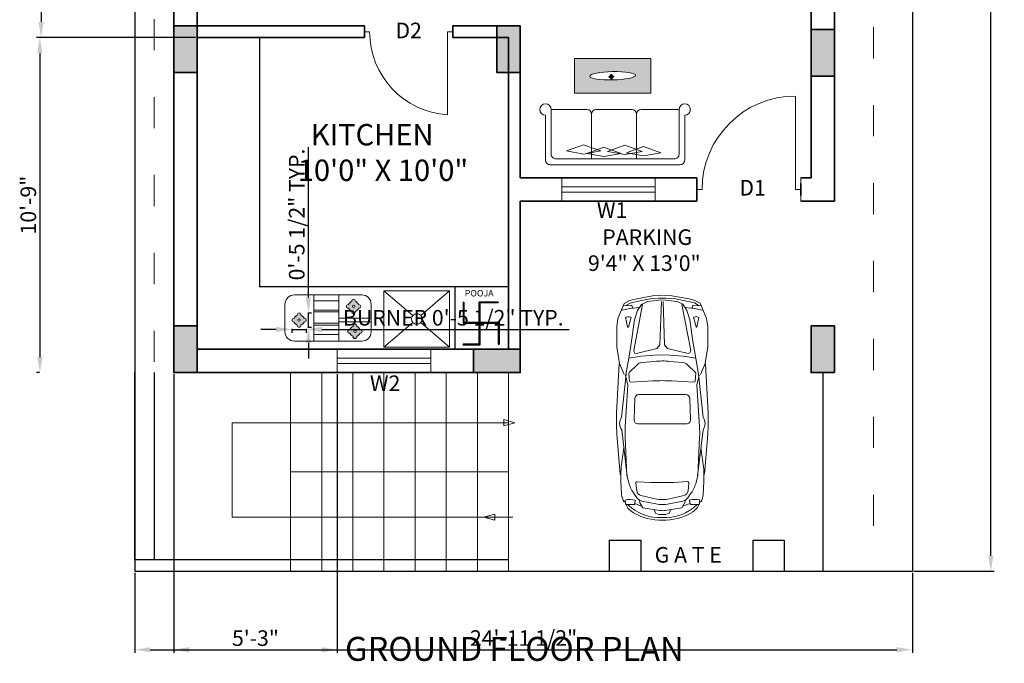
# Model space of a CAD drawing. Units: inches. Extents: x 40559 to 41508, y 131086 to 132358.
# Tile 1 of 5: x 40560 to 40939, y 131086 to 131334. Entities that reach past the tile are written whole.
import ezdxf

# ---------------------------------------------------------------- set-up
doc = ezdxf.new("R2010")
doc.units = ezdxf.units.IN
doc.linetypes.add('ACAD_ISO03W100', pattern=[30, 12, -18])
for name, color, linetype, lineweight in [('A-ANNO-DIMS', 2, 'Continuous', 18), ('A-ANNO-TEXT', 7, 'Continuous', 18), ('A-ANNO-TITL', 7, 'Continuous', 25), ('A-AREA-IDEN', 7, 'Continuous', 18), ('A-EQPM', 4, 'Continuous', 18), ('A-FLOR-CASE', 7, 'Continuous', 25), ('A-FLOR-FIXT', 4, 'Continuous', 18), ('A-FLOR-OVHD', 240, 'ACAD_ISO03W100', 13), ('A-FLOR-STRS', 240, 'Continuous', 18), ('A-FURN', 9, 'Continuous', 18), ('A-FURN-PATT', 252, 'Continuous', 13), ('A-SITE-VEHI', 9, 'Continuous', 13), ('A-SITE-WALL', 7, 'Continuous', 30), ('A-WALL', 7, 'Continuous', 35), ('C-PROP', 7, 'Continuous', 25), ('Doors', 50, 'Continuous', 18), ('Windows', 70, 'Continuous', 18)]:
    doc.layers.add(name, color=color, linetype=linetype, lineweight=lineweight)
doc.layers.add('A-COLS', color=177, linetype='Continuous', lineweight=35, true_color=0x293189)
doc.styles.get("Standard").update_dxf_attribs({"font": 'arial.ttf'})
doc.dimstyles.new('ISO-25', dxfattribs={"dimtxt": 6, "dimasz": 6, "dimexe": 1.25, "dimexo": 0.625, "dimtad": 1, "dimdec": 0, "dimlunit": 3, "dimtxsty": 'Standard', "dimcen": 2.5, "dimclrd": 1, "dimclre": 1, "dimclrt": 2, "dimadec": 0, "dimazin": 0, "dimtfac": 1, "dimtdec": 0, "dimtmove": 0, "dimatfit": 3, "dimfxl": 1, "dimarcsym": 0})

# ---------------------------------------------------------------- blocks, each defined once
blk = doc.blocks.new('*D10')
at = {"layer": 'A-ANNO-DIMS', "color": 0, "lineweight": -2, "transparency": 16777216}
for p, q in [((40618.81, 131457.85), (40567.14, 131457.85)), ((40568.39, 131451.85), (40568.39, 131333.35)), ((40627.81, 131327.35), (40567.14, 131327.35))]:
    blk.add_line(p, q, dxfattribs=at)
at = {"layer": 'A-ANNO-DIMS', "color": 0, "transparency": 16777216}
for points in [[(40567.39, 131451.85), (40569.39, 131451.85), (40568.39, 131457.85)], [(40567.39, 131333.35), (40569.39, 131333.35), (40568.39, 131327.35)]]:
    blk.add_solid(points, dxfattribs=at)
at = {"layer": 'Defpoints', "color": 0, "transparency": 16777216}
for p in [(40619.44, 131457.85), (40568.39, 131327.35), (40628.44, 131327.35)]:
    blk.add_point(p, dxfattribs=at)
at = {"layer": 'A-ANNO-DIMS', "color": 0, "transparency": 16777216, "insert": (40564.7, 131392.6), "char_height": 6, "attachment_point": 5, "rotation": 90}
blk.add_mtext('10\'-11"', dxfattribs=at)
blk = doc.blocks.new('*D6')
at = {"layer": 'A-ANNO-DIMS', "color": 0, "lineweight": -2, "transparency": 16777216}
for p, q in [((40567.76, 131327.35), (40566.65, 131327.35)), ((40567.9, 131321.35), (40567.9, 131204.35)), ((40567.76, 131198.35), (40566.65, 131198.35))]:
    blk.add_line(p, q, dxfattribs=at)
at = {"layer": 'A-ANNO-DIMS', "color": 0, "transparency": 16777216}
for points in [[(40566.9, 131321.35), (40568.9, 131321.35), (40567.9, 131327.35)], [(40566.9, 131204.35), (40568.9, 131204.35), (40567.9, 131198.35)]]:
    blk.add_solid(points, dxfattribs=at)
at = {"layer": 'Defpoints', "color": 0, "transparency": 16777216}
for p in [(40568.39, 131327.35), (40567.9, 131198.35), (40568.39, 131198.35)]:
    blk.add_point(p, dxfattribs=at)
at = {"layer": 'A-ANNO-DIMS', "color": 0, "transparency": 16777216, "insert": (40564.22, 131262.85), "char_height": 6, "attachment_point": 5, "rotation": 90}
blk.add_mtext('10\'-9"', dxfattribs=at)
blk = doc.blocks.new('WIN-36IN')
for p, q in [((0, 5.5), (36, 5.5)), ((0, 3.5), (36, 3.5))]:
    blk.add_line(p, q)
blk.add_lwpolyline([(0, 9), (36, 9), (36, 0), (0, 0)], close=True)
blk = doc.blocks.new('DOOR-KITCHEN-34IN')
for p, q in [((34, 29.75), (34, 34.25)), ((34, 29.75), (34, 34.25)), ((0, 32), (2, 32)), ((34, 32), (32, 32)), ((32, 32), (32, 0))]:
    blk.add_line(p, q)
blk.add_arc((34.07, 32), 32.07, 180, 266.3048)
blk = doc.blocks.new('DOOR-ENTRY-40IN')
for p, q in [((38, 4.5), (38, 40.5)), ((40, 9), (40, 0)), ((2, 4.5), (0, 4.5)), ((40, 4.5), (38, 4.5)), ((40, 6.75), (40, 2.25))]:
    blk.add_line(p, q)
blk.add_arc((38, 4.5), 36, 90, 180)
blk = doc.blocks.new('COL-9X18IN')
h = blk.add_hatch(color=256)
h.dxf.hatch_style = 1
h.paths.add_polyline_path([(9, 18), (0, 18), (0, 0), (9, 0)])
blk.add_lwpolyline([(0, 18), (9, 18), (9, 0), (0, 0)], close=True)
blk = doc.blocks.new('ENTRY-STAIR-PLAN')
for p, q in [((22.49, 76.5), (22.49, 0)), ((34.49, 76.5), (34.49, 0)), ((46.49, 76.5), (46.49, 0)), ((58.49, 76.5), (58.49, 0)), ((70.49, 76.5), (70.49, 0)), ((82.49, 76.5), (82.49, 0)), ((94.49, 76.5), (94.49, 0)), ((106.49, 76.5), (106.49, 0)), ((106.49, 57.22), (0, 57.22)), ((0, 57.22), (0, 20.84)), ((97.68, 57.22), (104.71, 57.22)), ((104.71, 57.22), (104.71, 58.4)), ((104.71, 58.4), (108.86, 57.22)), ((104.71, 57.22), (104.71, 56.03)), ((104.71, 56.03), (108.86, 57.22)), ((106.49, 38.25), (22.49, 38.25)), ((0, 20.84), (106.49, 20.84)), ((101.13, 22.03), (96.98, 20.84)), ((101.13, 19.65), (96.98, 20.84)), ((101.13, 20.84), (101.13, 22.03)), ((108.16, 20.84), (101.13, 20.84)), ((101.13, 20.84), (101.13, 19.65))]:
    blk.add_line(p, q)
blk = doc.blocks.new('GATE-PIER-12IN')
for p, q in [((0, 0), (0, 12)), ((0, 12), (12, 12)), ((0, 0), (0, 12)), ((0, 12), (12, 12)), ((12, 12), (12, 0)), ((12, 12), (12, 0))]:
    blk.add_line(p, q)
blk = doc.blocks.new('COOKTOP-BURNER')
h = blk.add_hatch(color=256)
h.dxf.hatch_style = 1
h.paths.add_polyline_path([(3.49, 4.67), (3.49, 4.81, 1), (2.04, 4.81), (2.04, 4.67, 0.214506), (0.86, 3.49), (0.72, 3.49, 1), (0.72, 2.04), (0.86, 2.04, 0.214506), (2.04, 0.86), (2.04, 0.72, 1), (3.49, 0.72), (3.49, 0.86, 0.214506), (4.67, 2.04), (4.81, 2.04, 1), (4.81, 3.49), (4.67, 3.49, 0.214506)])
h.paths.add_polyline_path([(3.21, 2.77, -1), (2.32, 2.77, -1)], flags=16)
for p, q in [((2.04, 4.81), (2.04, 4.67)), ((3.49, 4.81), (3.49, 4.67)), ((0.72, 3.49), (0.86, 3.49)), ((0.72, 2.04), (0.86, 2.04)), ((2.04, 0.86), (2.04, 0.72)), ((3.49, 0.86), (3.49, 0.72)), ((4.67, 3.49), (4.81, 3.49)), ((4.67, 2.04), (4.81, 2.04))]:
    blk.add_line(p, q)
blk.add_circle((2.77, 2.77), 0.442)
for centre, radius, start, end in [((2.77, 2.77), 2.04, 110.7864, 159.2136), ((2.77, 4.81), 0.724, 0, 180), ((2.77, 2.77), 2.04, 20.7864, 69.2136), ((0.72, 2.77), 0.724, 90, 270), ((2.77, 2.77), 2.04, 200.7864, 249.2136), ((2.77, 0.72), 0.724, 180, 0), ((2.77, 2.77), 2.04, 290.7864, 339.2136), ((4.81, 2.77), 0.724, 270, 90)]:
    blk.add_arc(centre, radius, start, end)
blk = doc.blocks.new('*D54')
at = {"layer": 'A-ANNO-DIMS', "color": 1, "lineweight": -2, "transparency": 16777216}
for p, q in [((40658.97, 131214.97), (40652.97, 131214.97)), ((40664.97, 131215.17), (40664.97, 131213.72)), ((40664.97, 131214.97), (40670.5, 131214.97)), ((40670.5, 131215.17), (40670.5, 131213.72)), ((40676.5, 131214.97), (40771.76, 131214.97))]:
    blk.add_line(p, q, dxfattribs=at)
at = {"layer": 'A-ANNO-DIMS', "color": 1, "transparency": 16777216}
for points in [[(40658.97, 131215.97), (40658.97, 131213.97), (40664.97, 131214.97)], [(40676.5, 131215.97), (40676.5, 131213.97), (40670.5, 131214.97)]]:
    blk.add_solid(points, dxfattribs=at)
at = {"layer": 'Defpoints', "color": 0, "transparency": 16777216}
for p in [(40664.97, 131215.8), (40670.5, 131215.8), (40670.5, 131214.97)]:
    blk.add_point(p, dxfattribs=at)
at = {"layer": 'A-ANNO-DIMS', "color": 2, "transparency": 16777216, "insert": (40727.13, 131218.69), "char_height": 6, "attachment_point": 5}
blk.add_mtext('BURNER 0\'-5 1/2" TYP.', dxfattribs=at)
blk = doc.blocks.new('*D55')
at = {"layer": 'A-ANNO-DIMS', "color": 1, "lineweight": -2, "transparency": 16777216}
for p, q in [((40671.33, 131227.32), (40671.33, 131285.13)), ((40671.12, 131221.32), (40672.58, 131221.32)), ((40671.33, 131215.8), (40671.33, 131221.32)), ((40671.12, 131215.8), (40672.58, 131215.8)), ((40671.33, 131209.8), (40671.33, 131203.8))]:
    blk.add_line(p, q, dxfattribs=at)
at = {"layer": 'A-ANNO-DIMS', "color": 1, "transparency": 16777216}
for points in [[(40670.33, 131227.32), (40672.33, 131227.32), (40671.33, 131221.32)], [(40670.33, 131209.8), (40672.33, 131209.8), (40671.33, 131215.8)]]:
    blk.add_solid(points, dxfattribs=at)
at = {"layer": 'Defpoints', "color": 0, "transparency": 16777216}
for p in [(40670.5, 131221.32), (40671.33, 131221.32), (40670.5, 131215.8)]:
    blk.add_point(p, dxfattribs=at)
at = {"layer": 'A-ANNO-DIMS', "color": 2, "transparency": 16777216, "insert": (40667.6, 131259.23), "char_height": 6, "attachment_point": 5, "rotation": 90}
blk.add_mtext('0\'-5 1/2" TYP.', dxfattribs=at)
blk = doc.blocks.new('*D64')
at = {"layer": 'A-ANNO-DIMS', "color": 1, "lineweight": -2, "transparency": 16777216}
for p, q in [((40604.44, 131121.23), (40604.44, 131090.4)), ((40903.94, 131121.23), (40903.94, 131090.4)), ((40610.44, 131091.65), (40897.94, 131091.65))]:
    blk.add_line(p, q, dxfattribs=at)
at = {"layer": 'A-ANNO-DIMS', "color": 1, "transparency": 16777216}
for points in [[(40610.44, 131092.65), (40610.44, 131090.65), (40604.44, 131091.65)], [(40897.94, 131092.65), (40897.94, 131090.65), (40903.94, 131091.65)]]:
    blk.add_solid(points, dxfattribs=at)
at = {"layer": 'Defpoints', "color": 0, "transparency": 16777216}
for p in [(40604.44, 131121.85), (40903.94, 131121.85), (40903.94, 131091.65)]:
    blk.add_point(p, dxfattribs=at)
at = {"layer": 'A-ANNO-DIMS', "color": 2, "transparency": 16777216, "insert": (40754.19, 131095.38), "char_height": 6, "attachment_point": 5}
blk.add_mtext('24\'-11 1/2"', dxfattribs=at)
blk = doc.blocks.new('*D65')
at = {"layer": 'A-ANNO-DIMS', "color": 1, "lineweight": -2, "transparency": 16777216}
for p, q in [((40904.56, 131667.35), (40935.39, 131667.35)), ((40934.14, 131127.85), (40934.14, 131661.35)), ((40904.56, 131121.85), (40935.39, 131121.85))]:
    blk.add_line(p, q, dxfattribs=at)
at = {"layer": 'A-ANNO-DIMS', "color": 1, "transparency": 16777216}
for points in [[(40933.14, 131661.35), (40935.14, 131661.35), (40934.14, 131667.35)], [(40933.14, 131127.85), (40935.14, 131127.85), (40934.14, 131121.85)]]:
    blk.add_solid(points, dxfattribs=at)
at = {"layer": 'Defpoints', "color": 0, "transparency": 16777216}
for p in [(40903.94, 131667.35), (40934.14, 131667.35), (40903.94, 131121.85)]:
    blk.add_point(p, dxfattribs=at)
at = {"layer": 'A-ANNO-DIMS', "color": 2, "transparency": 16777216, "insert": (40930.41, 131394.6), "char_height": 6, "attachment_point": 5, "rotation": 90}
blk.add_mtext('45\'-5 1/2"', dxfattribs=at)
blk = doc.blocks.new('*D70')
at = {"layer": 'A-ANNO-DIMS', "color": 1, "lineweight": -2, "transparency": 16777216}
for p, q in [((40619.44, 131197.73), (40619.44, 131090.4)), ((40682.44, 131197.73), (40682.44, 131090.4)), ((40625.44, 131091.65), (40676.44, 131091.65))]:
    blk.add_line(p, q, dxfattribs=at)
at = {"layer": 'A-ANNO-DIMS', "color": 1, "transparency": 16777216}
for points in [[(40625.44, 131092.65), (40625.44, 131090.65), (40619.44, 131091.65)], [(40676.44, 131092.65), (40676.44, 131090.65), (40682.44, 131091.65)]]:
    blk.add_solid(points, dxfattribs=at)
at = {"layer": 'Defpoints', "color": 0, "transparency": 16777216}
for p in [(40619.44, 131198.35), (40682.44, 131198.35), (40682.44, 131091.65)]:
    blk.add_point(p, dxfattribs=at)
at = {"layer": 'A-ANNO-DIMS', "color": 2, "transparency": 16777216, "insert": (40650.94, 131095.34), "char_height": 6, "attachment_point": 5}
blk.add_mtext('5\'-3"', dxfattribs=at)

msp = doc.modelspace()

# ---------------------------------------------------------------- hatches: boundary and pattern name
at = {"layer": 'A-FURN-PATT'}
h = msp.add_hatch(color=256, dxfattribs=at)
h.dxf.hatch_style = 1
h.paths.add_polyline_path([(40803.17, 131319.32), (40773.78, 131319.32), (40773.78, 131305.95), (40803.17, 131305.95)])
edge = h.paths.add_edge_path(flags=16)
edge.add_ellipse((40788.51, 131312.63), major_axis=(-8.8, -0.18), ratio=0.181718, start_angle=0, end_angle=360)
h = msp.add_hatch(color=256, dxfattribs=at)
h.dxf.hatch_style = 1
edge = h.paths.add_edge_path()
edge.add_ellipse((40788, 131312.29), major_axis=(-0.977, -0.018), ratio=0.42283, start_angle=498.0011, end_angle=228.0011)
edge.add_ellipse((40788, 131312.29), major_axis=(-0.12, 0.969), ratio=0.42283, start_angle=311.9989, end_angle=401.9989)
edge.add_ellipse((40788, 131312.29), major_axis=(-0.977, -0.018), ratio=0.42283, start_angle=318.0011, end_angle=408.0011)
edge.add_ellipse((40788, 131312.29), major_axis=(-0.12, 0.969), ratio=0.42283, start_angle=131.9989, end_angle=221.9989)
h = msp.add_hatch(color=256, dxfattribs=at)
h.dxf.hatch_style = 1
h.paths.add_polyline_path([(40744.74, 131217.72), (40737.31, 131217.72), (40737.31, 131225.17), (40744.42, 131225.17), (40744.42, 131225.5), (40736.98, 131225.5), (40736.98, 131217.72), (40731.24, 131217.72), (40731.24, 131223.03), (40731.24, 131225.5), (40730.92, 131225.5), (40730.92, 131223.03), (40730.92, 131217.39), (40736.98, 131217.39), (40736.98, 131209.29), (40730.92, 131209.29), (40730.92, 131208.96), (40737.31, 131208.96), (40737.31, 131217.39), (40744.42, 131217.39), (40744.42, 131210.6), (40744.42, 131209.29), (40744.74, 131209.29), (40744.74, 131210.6)])

# ---------------------------------------------------------------- linework, layer by layer
at = {"layer": 'A-EQPM'}
for p, q in [((40665.93, 131228.27), (40691.88, 131228.27)), ((40673.45, 131219.36), (40673.45, 131228.27)), ((40673.45, 131228.27), (40673.45, 131210.45)), ((40673.45, 131226.04), (40683.11, 131226.04)), ((40683.11, 131228.27), (40683.11, 131210.45)), ((40662.31, 131214.07), (40662.31, 131224.65)), ((40673.45, 131222.42), (40683.11, 131222.42)), ((40673.45, 131221.7), (40683.11, 131221.7)), ((40695.5, 131224.65), (40695.5, 131214.07)), ((40695.5, 131219.36), (40683.11, 131219.36)), ((40683.11, 131217.91), (40695.5, 131217.91)), ((40673.45, 131217.35), (40683.11, 131217.35)), ((40673.45, 131216.63), (40683.11, 131216.63)), ((40691.88, 131210.45), (40665.93, 131210.45)), ((40673.45, 131213), (40683.11, 131213))]:
    msp.add_line(p, q, dxfattribs=at)
for centre, start, end in [((40665.93, 131224.65), 90, 180), ((40691.88, 131224.65), 0, 90), ((40665.93, 131214.07), 180, 270), ((40691.88, 131214.07), 270, 0)]:
    msp.add_arc(centre, 3.62, start, end, dxfattribs=at)
at = {"layer": 'A-FLOR-CASE'}
for p, q in [((40652.44, 131327.35), (40652.44, 131231.35)), ((40748.44, 131231.35), (40652.44, 131231.35)), ((40727.76, 131231.35), (40727.76, 131207.35)), ((40730.92, 131225.5), (40731.24, 131225.5)), ((40744.42, 131225.5), (40744.42, 131225.17)), ((40730.92, 131209.29), (40730.92, 131208.96)), ((40744.42, 131209.29), (40744.74, 131209.29))]:
    msp.add_line(p, q, dxfattribs=at)
for points in [[(40730.92, 131225.5), (40730.92, 131223.03), (40730.92, 131217.39), (40736.98, 131217.39)], [(40731.24, 131225.5), (40731.24, 131223.03), (40731.24, 131217.72), (40736.98, 131217.72)], [(40744.42, 131225.5), (40736.98, 131225.5), (40736.98, 131217.72)], [(40744.42, 131225.17), (40737.31, 131225.17), (40737.31, 131217.72)], [(40736.98, 131217.39), (40736.98, 131209.29), (40730.92, 131209.29)], [(40737.31, 131217.39), (40737.31, 131208.96), (40730.92, 131208.96)], [(40737.31, 131217.72), (40744.74, 131217.72), (40744.74, 131210.6), (40744.74, 131209.29)], [(40737.31, 131217.39), (40744.42, 131217.39), (40744.42, 131210.6), (40744.42, 131209.29)]]:
    msp.add_lwpolyline(points, dxfattribs=at)
at = {"layer": 'A-FLOR-FIXT'}
for p, q in [((40700.44, 131229.84), (40711.53, 131220.34)), ((40725.72, 131229.84), (40714.64, 131220.34)), ((40711.53, 131217.67), (40700.44, 131208.17)), ((40714.64, 131217.67), (40725.72, 131208.17))]:
    msp.add_line(p, q, dxfattribs=at)
msp.add_lwpolyline([(40700.44, 131229.84), (40725.72, 131229.84), (40725.72, 131208.17), (40700.44, 131208.17)], close=True, dxfattribs=at)
msp.add_circle((40713.08, 131219.01), 2.05, dxfattribs=at)
at = {"layer": 'A-FLOR-OVHD'}
for p, q in [((40611.94, 131202.46), (40611.94, 131661.35)), ((40888.94, 131661.35), (40888.94, 131121.85))]:
    msp.add_line(p, q, dxfattribs=at)
at = {"layer": 'A-FURN'}
for p, q in [((40764.85, 131299.63), (40778.56, 131299.63)), ((40780.38, 131297.81), (40780.38, 131280.6)), ((40782.21, 131299.63), (40795.87, 131299.63)), ((40797.69, 131297.81), (40797.69, 131280.6)), ((40814.09, 131299.63), (40799.52, 131299.63)), ((40777.34, 131286.09), (40770.72, 131283.68)), ((40777.34, 131286.09), (40783.96, 131283.68)), ((40770.72, 131283.68), (40777.34, 131282.51)), ((40783.96, 131283.68), (40777.34, 131282.51)), ((40785.13, 131285.12), (40778.51, 131282.71)), ((40778.51, 131282.71), (40785.13, 131281.54)), ((40785.13, 131285.12), (40791.75, 131282.71)), ((40791.75, 131282.71), (40785.13, 131281.54)), ((40793.2, 131285.95), (40786.58, 131283.54)), ((40786.58, 131283.54), (40793.2, 131282.37)), ((40793.2, 131285.95), (40799.82, 131283.54)), ((40799.82, 131283.54), (40793.2, 131282.37)), ((40800.44, 131285.39), (40793.82, 131282.98)), ((40793.82, 131282.98), (40800.44, 131281.82)), ((40800.44, 131285.39), (40807.06, 131282.98)), ((40807.06, 131282.98), (40800.44, 131281.82))]:
    msp.add_line(p, q, dxfattribs=at)
msp.add_lwpolyline([(40773.78, 131319.32), (40803.17, 131319.32), (40803.17, 131305.95), (40773.78, 131305.95)], close=True, dxfattribs=at)
for points in [[(40814.09, 131299.63), (40814.09, 131282.42, -0.414214), (40812.26, 131280.6), (40766.68, 131280.6, -0.414214), (40764.85, 131282.42), (40764.85, 131299.63)], [(40816.28, 131297.44), (40816.28, 131280.23, -0.414214), (40814.46, 131278.4), (40764.49, 131278.4, -0.414214), (40762.66, 131280.23), (40762.66, 131297.44)]]:
    msp.add_lwpolyline(points, format="xyb", dxfattribs=at)
for centre, radius, start, end in [((40762.66, 131299.63), 2.19, 0, 270), ((40816.28, 131299.63), 2.19, 270, 180), ((40778.56, 131297.81), 1.83, 0, 90), ((40782.21, 131297.81), 1.83, 90, 180), ((40795.87, 131297.81), 1.83, 0, 90), ((40799.52, 131297.81), 1.83, 90, 180)]:
    msp.add_arc(centre, radius, start, end, dxfattribs=at)
msp.add_ellipse((40788.51, 131312.63), major_axis=(-8.8, -0.18), ratio=0.181718, dxfattribs=at)
for major_axis, start_param, end_param in [((-0.977, -0.018), 5.151437, 7.490221), ((-0.12, 0.969), 5.07615, 7.414933), ((-0.977, -0.018), 8.29303, 10.631813), ((-0.12, 0.969), 1.934557, 4.27334)]:
    msp.add_ellipse((40788, 131312.29), major_axis=major_axis, ratio=0.42283, start_param=start_param, end_param=end_param, dxfattribs=at)
at = {"layer": 'A-SITE-VEHI'}
for p, q in [((40799.46, 131226.1), (40795.22, 131225.14)), ((40802.97, 131226.82), (40799.46, 131226.1)), ((40806.23, 131227), (40802.97, 131226.82)), ((40808.98, 131227.01), (40812.24, 131226.83)), ((40812.24, 131226.83), (40815.75, 131226.12)), ((40815.75, 131226.12), (40820, 131225.16)), ((40792.07, 131222.4), (40792.69, 131222.55)), ((40795.85, 131224.32), (40792.87, 131224.07)), ((40795.22, 131225.14), (40793.41, 131224.07)), ((40796.11, 131223.15), (40795.85, 131224.32)), ((40797.63, 131223.3), (40798.65, 131223.37)), ((40817.59, 131223.32), (40816.57, 131223.39)), ((40819.11, 131223.18), (40819.37, 131224.34)), ((40819.37, 131224.34), (40822.35, 131224.1)), ((40820, 131225.16), (40821.8, 131224.1)), ((40823.16, 131222.43), (40822.53, 131222.58)), ((40794.22, 131219.81), (40793.51, 131219.55)), ((40793.51, 131219.55), (40794.29, 131215.92)), ((40794.59, 131215.91), (40795.59, 131219.68)), ((40795.59, 131219.68), (40794.8, 131219.85)), ((40819.64, 131219.7), (40820.42, 131219.88)), ((40820.64, 131215.94), (40819.64, 131219.7)), ((40821.71, 131219.58), (40820.95, 131215.95)), ((40821.01, 131219.84), (40821.71, 131219.58)), ((40793.64, 131197.58), (40794.7, 131203.89)), ((40804.67, 131202.68), (40799.79, 131202.22)), ((40810.59, 131202.69), (40815.46, 131202.23)), ((40821.62, 131197.61), (40820.55, 131203.92)), ((40790.96, 131201.75), (40790.03, 131182.84)), ((40797.89, 131201.32), (40794.89, 131198.35)), ((40817.36, 131201.34), (40820.37, 131198.37)), ((40824.29, 131201.78), (40825.26, 131182.87)), ((40793.72, 131197.73), (40791.96, 131181.18)), ((40793.47, 131197.34), (40794.33, 131193.58)), ((40794.74, 131197.94), (40794.96, 131195.12)), ((40795.51, 131194.64), (40804, 131195.15)), ((40819.76, 131194.67), (40811.27, 131195.15)), ((40820.52, 131197.96), (40820.31, 131195.15)), ((40821.8, 131197.37), (40820.94, 131193.6)), ((40821.54, 131197.76), (40823.34, 131181.21)), ((40794.33, 131193.58), (40793.34, 131177.49)), ((40820.94, 131193.6), (40821.96, 131177.52)), ((40797.04, 131188.35), (40796.79, 131180.2)), ((40798.6, 131189.87), (40816.68, 131189.89)), ((40818.24, 131188.38), (40818.5, 131180.22)), ((40791.99, 131176.33), (40794.14, 131158.53)), ((40816.94, 131178.61), (40798.36, 131178.59)), ((40823.31, 131176.36), (40821.2, 131158.55)), ((40790.16, 131174.61), (40791.44, 131159.15)), ((40793.31, 131173.52), (40793.97, 131158.75)), ((40822, 131173.54), (40821.37, 131158.78)), ((40825.14, 131174.65), (40823.9, 131159.19)), ((40792.86, 131169.52), (40792.04, 131163.87)), ((40822.46, 131169.55), (40823.29, 131163.9)), ((40793.97, 131158.75), (40794.7, 131156)), ((40821.37, 131158.78), (40820.65, 131156.03)), ((40791.71, 131156.45), (40791.98, 131151.45)), ((40797.45, 131155.77), (40797.8, 131152.82)), ((40798, 131156.35), (40803.26, 131156.08)), ((40803.26, 131156.08), (40807.64, 131156.09)), ((40812.08, 131156.08), (40807.71, 131156.09)), ((40817.35, 131156.37), (40812.08, 131156.08)), ((40817.89, 131155.79), (40817.55, 131152.84)), ((40823.64, 131156.48), (40823.38, 131151.48)), ((40796.55, 131152.03), (40797.85, 131150.17)), ((40799.4, 131151.04), (40804.85, 131149.78)), ((40815.95, 131151.05), (40810.5, 131149.78)), ((40818.81, 131152.05), (40817.5, 131150.18)), ((40793.2, 131148.68), (40793.48, 131148.02)), ((40793.44, 131147.83), (40793.34, 131149.29)), ((40796.75, 131147.59), (40793.7, 131147.58)), ((40793.7, 131147.5), (40793.96, 131146.88)), ((40797.24, 131149.22), (40797, 131147.81)), ((40797.01, 131148), (40799.86, 131146.86)), ((40798.81, 131149.27), (40799, 131148.27)), ((40799, 131148.27), (40800.19, 131146.32)), ((40799.78, 131148.9), (40805.14, 131147.79)), ((40800.19, 131146.32), (40806.67, 131145.27)), ((40815.18, 131146.34), (40808.7, 131145.27)), ((40815.58, 131148.91), (40810.22, 131147.8)), ((40816.36, 131148.28), (40815.18, 131146.34)), ((40818.35, 131148.02), (40815.5, 131146.87)), ((40816.55, 131149.29), (40816.36, 131148.28)), ((40818.12, 131149.24), (40818.36, 131147.83)), ((40818.61, 131147.61), (40821.66, 131147.61)), ((40821.66, 131147.52), (40821.4, 131146.91)), ((40822.16, 131148.71), (40821.88, 131148.04)), ((40821.92, 131147.86), (40822.01, 131149.32)), ((40804.49, 131145.6), (40805.06, 131144.25)), ((40805.06, 131144.25), (40806.34, 131143.75)), ((40806.34, 131143.75), (40807.68, 131143.68)), ((40809.03, 131143.76), (40807.69, 131143.68)), ((40810.31, 131144.26), (40809.03, 131143.76)), ((40810.88, 131145.6), (40810.31, 131144.26))]:
    msp.add_line(p, q, dxfattribs=at)
for points in [[(40807.4, 131228.02), (40803.87, 131227.9), (40797.29, 131226.69), (40795.03, 131226.09), (40792.96, 131225.02), (40790.53, 131219.2), (40790.09, 131215.98), (40790.1, 131208.27), (40791.1, 131201.85), (40792.92, 131197.58)], [(40807.48, 131226.31), (40801.9, 131225.72), (40799.64, 131224.63), (40798.12, 131222.26), (40796.94, 131218.63), (40795.66, 131209.51), (40794.7, 131203.89), (40799.55, 131204.67), (40804.64, 131205.08), (40807.62, 131205.26)], [(40800.06, 131224.55), (40796.61, 131206.87), (40796.98, 131205.89), (40797.71, 131205.72), (40805.56, 131207.65), (40806.72, 131209.06), (40807.29, 131225.79)], [(40807.73, 131226.31), (40813.31, 131225.73), (40815.58, 131224.64), (40817.1, 131222.27), (40818.29, 131218.65), (40819.58, 131209.54), (40820.55, 131203.92), (40815.7, 131204.69), (40810.61, 131205.08), (40807.62, 131205.26)], [(40807.81, 131228.02), (40811.34, 131227.91), (40817.92, 131226.71), (40820.18, 131226.12), (40822.25, 131225.05), (40824.7, 131219.23), (40825.15, 131216.02), (40825.15, 131208.3), (40824.15, 131201.89), (40822.35, 131197.61)], [(40815.16, 131224.57), (40818.63, 131206.89), (40818.26, 131205.92), (40817.54, 131205.74), (40809.68, 131207.66), (40808.52, 131209.06), (40807.92, 131225.79)]]:
    msp.add_lwpolyline(points, dxfattribs=at)
for centre, radius, start, end in [((40807.63, 131202.04), 25, 86.8942, 93.2188), ((40799.83, 131192.13), 31.25, 94.0319, 103.1964), ((40815.45, 131192.14), 31.25, 76.9166, 86.0811), ((40794.58, 131218.83), 1.04, 77.5746, 110.1342), ((40820.65, 131218.86), 1.04, 69.9787, 102.5384), ((40794.44, 131215.95), 0.156, 192.0005, 345.153), ((40820.79, 131215.98), 0.156, 194.96, 348.1125), ((40807.66, 131171.58), 31.25, 84.6214, 95.4916), ((40800.09, 131199.11), 3.12, 95.4916, 134.8083), ((40815.17, 131199.12), 3.12, 45.3046, 84.6214), ((40795.26, 131197.98), 0.521, 134.8083, 184.3979), ((40795.48, 131195.16), 0.521, 184.3979, 273.3874), ((40807.7, 131132.75), 62.5, 86.7256, 93.3874), ((40819.79, 131195.19), 0.521, 266.7256, 355.7151), ((40820, 131198), 0.521, 355.7151, 45.3046), ((40798.6, 131188.31), 1.56, 90.1141, 178.2929), ((40816.68, 131188.33), 1.56, 1.8201, 89.9989), ((40852.45, 131179.75), 62.5, 177.1678, 184.7177), ((40795.43, 131178.78), 4.23, 145.336, 215.4638), ((40798.36, 131180.15), 1.56, 178.2929, 270.1885), ((40816.94, 131180.17), 1.56, 269.9245, 1.8201), ((40819.87, 131178.8), 4.23, 324.6492, 34.7769), ((40762.85, 131179.66), 62.5, 355.3952, 2.9452), ((40830.77, 131175.19), 37.5, 176.4893, 182.5638), ((40784.54, 131175.15), 37.5, 357.5491, 3.6237), ((40829.15, 131158.49), 37.5, 171.7454, 183.1132), ((40786.19, 131158.45), 37.5, 356.9998, 8.3676), ((40806.78, 131159.21), 12.5, 194.8579, 215.0429), ((40797.97, 131155.83), 0.521, 86.9979, 186.737), ((40817.37, 131155.85), 0.521, 353.376, 93.115), ((40808.56, 131159.21), 12.5, 325.07, 345.2551), ((40797.8, 131151.74), 5.83, 182.9306, 212.783), ((40799.87, 131153.07), 2.08, 186.737, 256.9903), ((40800.41, 131151.96), 3.12, 215.0429, 258.3436), ((40807.67, 131161.96), 12.5, 256.9903, 283.1226), ((40814.94, 131151.97), 3.12, 281.7694, 325.07), ((40815.48, 131153.08), 2.08, 283.1226, 353.376), ((40817.55, 131151.76), 5.83, 327.3299, 357.1824), ((40795.15, 131142.05), 7.46, 73.7595, 104.0169), ((40793.7, 131147.84), 0.26, 183.7825, 270.113), ((40796.84, 131148.1), 3.12, 202.9116, 223.7293), ((40806.51, 131159.92), 17.38, 225.5935, 273.8679), ((40801.04, 131152.11), 8.93, 223.7293, 239.6553), ((40796.75, 131147.85), 0.26, 270.113, 350.5053), ((40807.67, 131160.03), 12.5, 258.3436, 281.7694), ((40808.83, 131159.92), 17.38, 266.2451, 314.5195), ((40820.22, 131142.08), 7.46, 76.0961, 106.3535), ((40818.61, 131147.87), 0.26, 189.6077, 270), ((40814.32, 131152.13), 8.93, 300.4577, 316.3836), ((40818.52, 131148.12), 3.12, 316.3836, 337.2014), ((40821.66, 131147.87), 0.26, 270, 356.3304), ((40807.01, 131162.31), 20.75, 239.6553, 272.0435), ((40807.68, 131151.43), 6.25, 260.7246, 279.3883), ((40808.33, 131162.31), 20.75, 268.0694, 300.4577)]:
    msp.add_arc(centre, radius, start, end, dxfattribs=at)
at = {"layer": 'A-SITE-WALL'}
for p, q in [((40604.44, 131126.35), (40604.44, 131198.35)), ((40611.94, 131198.35), (40611.94, 131126.35)), ((40869.44, 131198.35), (40869.44, 131121.85)), ((40604.44, 131126.35), (40748.44, 131126.35)), ((40604.44, 131121.85), (40748.44, 131121.85))]:
    msp.add_line(p, q, dxfattribs=at)
at = {"layer": 'A-WALL'}
for p, q in [((40619.44, 131655.35), (40619.44, 131198.35)), ((40873.94, 131655.35), (40873.94, 131264.35)), ((40628.44, 131646.35), (40628.44, 131207.35)), ((40864.94, 131646.35), (40864.94, 131273.35)), ((40628.44, 131331.85), (40692.9, 131331.85)), ((40692.9, 131327.35), (40692.9, 131331.85)), ((40726.9, 131331.85), (40752.94, 131331.85)), ((40726.9, 131327.35), (40726.9, 131331.85)), ((40752.94, 131331.85), (40752.94, 131273.35)), ((40628.44, 131327.35), (40692.9, 131327.35)), ((40628.44, 131327.35), (40628.44, 131207.35)), ((40726.9, 131327.35), (40748.44, 131327.35)), ((40748.44, 131327.35), (40748.44, 131207.35)), ((40752.94, 131273.35), (40820.94, 131273.35)), ((40820.94, 131273.35), (40820.94, 131264.35)), ((40860.94, 131273.35), (40864.94, 131273.35)), ((40860.94, 131271.1), (40860.94, 131266.6)), ((40752.94, 131264.35), (40820.94, 131264.35)), ((40752.94, 131264.35), (40752.94, 131198.35)), ((40860.94, 131264.35), (40873.94, 131264.35)), ((40628.44, 131207.35), (40748.44, 131207.35)), ((40619.44, 131198.35), (40752.94, 131198.35))]:
    msp.add_line(p, q, dxfattribs=at)
at = {"layer": 'C-PROP'}
for p, q in [((40604.44, 131667.35), (40604.44, 131121.85)), ((40903.94, 131667.35), (40903.94, 131121.85)), ((40604.44, 131121.85), (40903.94, 131121.85))]:
    msp.add_line(p, q, dxfattribs=at)

# ---------------------------------------------------------------- block references
at = {"layer": 'A-COLS'}
for p in [(40619.44, 131313.85), (40619.44, 131198.35)]:
    msp.add_blockref('COL-9X18IN', p, dxfattribs=at)
for p, rotation in [((40752.94, 131331.85), 180), ((40873.94, 131330.51), 180), ((40873.94, 131216.35), 180), ((40734.94, 131207.35), 270.0000000000411)]:
    msp.add_blockref('COL-9X18IN', p, dxfattribs=dict(at, rotation=rotation))
at = {"layer": 'A-EQPM'}
for p in [(40685.95, 131221.06), (40664.97, 131215.79), (40686.47, 131211.47)]:
    msp.add_blockref('COOKTOP-BURNER', p, dxfattribs=at)
at = {"layer": 'A-FLOR-STRS'}
msp.add_blockref('ENTRY-STAIR-PLAN', (40641.95, 131121.85), dxfattribs=at)
at = {"layer": 'A-SITE-WALL'}
for p in [(40787.33, 131121.85), (40842.57, 131121.85)]:
    msp.add_blockref('GATE-PIER-12IN', p, dxfattribs=at)
at = {"layer": 'Doors'}
for name, p in [('DOOR-KITCHEN-34IN', (40692.9, 131297.6)), ('DOOR-ENTRY-40IN', (40820.94, 131264.35))]:
    msp.add_blockref(name, p, dxfattribs=at)
at = {"layer": 'Windows'}
for p in [(40768.94, 131264.35), (40682.44, 131198.35)]:
    msp.add_blockref('WIN-36IN', p, dxfattribs=at)

# ---------------------------------------------------------------- texts
at = {"layer": 'A-ANNO-TEXT', "char_height": 6, "attachment_point": 1}
for s, width, insert in [('{D2}', 6, (40704.85, 131333.08)), ('{D1}', 6, (40837.33, 131272.54)), ('{W1}', 21.3561, (40782.42, 131263.91)), ('{W2}', 21.3561, (40695.01, 131197.26)), ('{\\fArial|b1|i0|c0|p34;G A T E}', 37.8561, (40804.71, 131131.19))]:
    msp.add_mtext_dynamic_manual_height_columns(s, width=width, gutter_width=12.5, heights=[0], dxfattribs=dict(at, insert=insert))
at = {"layer": 'A-ANNO-TITL', "insert": (40685.45, 131096.6), "char_height": 9.2211, "attachment_point": 1}
msp.add_mtext_dynamic_manual_height_columns('{\\fArial|b1|i0|c0|p34;GROUND FLOOR PLAN}', width=193.072, gutter_width=19.21, heights=[0], dxfattribs=at)
at = {"layer": 'A-AREA-IDEN', "attachment_point": 1}
for s, width, gutter_width, insert, char_height in [('{\\fArial|b1|i0|c0|p34;  KITCHEN\\P10\'0" X 10\'0"}', 121.5689, 17.12, (40667.23, 131294.06), 8.2185), ('{\\fArial|b1|i0|c0|p34;   PARKING\\P9\'4" X 13\'0"}', 54.4487, 12.5, (40779.01, 131253.5), 6), ('{\\fArial|b1|i0|c0|p34;POOJA}', 12.705, 12.5, (40731.54, 131230.17), 2.5)]:
    msp.add_mtext_dynamic_manual_height_columns(s, width=width, gutter_width=gutter_width, heights=[0], dxfattribs=dict(at, insert=insert, char_height=char_height))

# ---------------------------------------------------------------- dimensions: what is measured, and where the dimension line sits
at = {"layer": 'A-ANNO-DIMS'}
for base, p1, p2, override, picture, middle in [((40934.14, 131667.35), (40903.94, 131121.85), (40903.94, 131667.35), {"dimdec": 1, "dimlfac": 1, "dimrnd": 0, "dimzin": 1, "dimdsep": 46, "dimlunit": 4, "dimfrac": 2}, '*D65', (40930.41, 131394.6)), ((40568.38636267, 131327.35041044), (40619.43804113, 131457.85041044), (40628.43804113, 131327.35041044), {"dimclrd": 0, "dimclre": 0, "dimclrt": 0}, '*D10', (40564.69792474, 131392.60041044)), ((40567.9, 131198.35), (40568.39, 131327.35), (40568.39, 131198.35), {"dimclrd": 0, "dimclre": 0, "dimclrt": 0}, '*D6', (40564.22, 131262.85))]:
    dim = msp.add_linear_dim(base=base, p1=p1, p2=p2, angle=90, dimstyle='ISO-25', override=override, dxfattribs=at)
    dim.commit()
    dim.dimension.update_dxf_attribs({"geometry": picture, "text_midpoint": middle})
dim = msp.add_linear_dim(base=(40671.33, 131221.32), p1=(40670.5, 131215.8), p2=(40670.5, 131221.32), angle=90, text='<> TYP.', dimstyle='ISO-25', override={"dimdec": 1, "dimlfac": 1, "dimrnd": 0, "dimzin": 1, "dimdsep": 46, "dimlunit": 4, "dimfrac": 2}, dxfattribs=at)
dim.commit()
dim.dimension.update_dxf_attribs({"geometry": '*D55', "text_midpoint": (40667.6, 131259.23)})
dim = msp.add_linear_dim(base=(40670.5, 131214.97), p1=(40664.97, 131215.8), p2=(40670.5, 131215.8), text='BURNER <> TYP.', dimstyle='ISO-25', override={"dimdec": 1, "dimlfac": 1, "dimrnd": 0, "dimzin": 1, "dimdsep": 46, "dimlunit": 4, "dimfrac": 2}, dxfattribs=at)
dim.commit()
dim.dimension.update_dxf_attribs({"geometry": '*D54', "text_midpoint": (40727.13, 131218.69)})
for base, p1, p2, picture, middle in [((40682.44, 131091.65), (40619.44, 131198.35), (40682.44, 131198.35), '*D70', (40650.94, 131095.34)), ((40903.94, 131091.65), (40604.44, 131121.85), (40903.94, 131121.85), '*D64', (40754.19, 131095.38))]:
    dim = msp.add_linear_dim(base=base, p1=p1, p2=p2, dimstyle='ISO-25', override={"dimdec": 1, "dimlfac": 1, "dimrnd": 0, "dimzin": 1, "dimdsep": 46, "dimlunit": 4, "dimfrac": 2}, dxfattribs=at)
    dim.commit()
    dim.dimension.update_dxf_attribs({"geometry": picture, "text_midpoint": middle})

doc.saveas('drawing.dxf')
